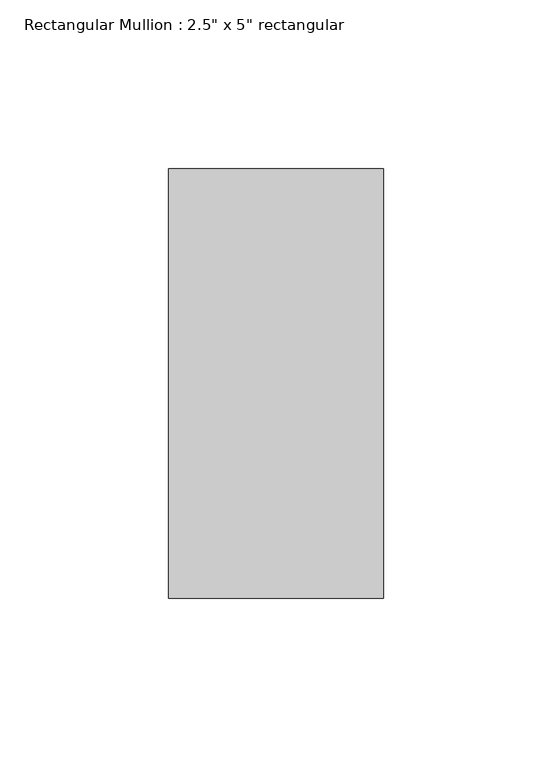
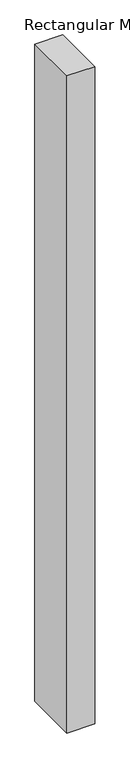
"""IFC4 building model written with IfcOpenShell, lengths in millimetres: member geometry."""

from ifc_helpers import new_model, si_unit, frame, origin, place, context, project, spatial, polyline, outline, extrude, source, transform, mapped, element, save


def member_46fa6ebc(model_context):
    return source(origin(), model_context, "Body", "SweptSolid", [
        extrude(outline(polyline([(31.75, 63.5), (31.75, -63.5), (-31.75, -63.5), (-31.75, 63.5), (31.75, 63.5)])), frame((0.0, 0.0, -1588.1134655), z_axis=(0.0, 0.0, 1.0), x_axis=(1.0, 0.0, 0.0)), (0.0, 0.0, 1.0), 1588.1134655),
    ])


if __name__ == "__main__":
    model = new_model("IFC4")
    model_context = context("Model", 3, world=origin())
    ifc_project = project(units=[si_unit("LENGTHUNIT", "METRE", prefix="MILLI")], contexts=[model_context])
    site = spatial("IfcSite", under=ifc_project)
    building = spatial("IfcBuilding", under=site)
    placement = place(None, origin())
    member_shape = member_46fa6ebc(model_context)
    element("IfcMember", 1, ObjectType="Rectangular Mullion : 2.5\" x 5\" rectangular", at=placement, inside=building, context=model_context, shape_type="MappedRepresentation", body=[
        mapped(member_shape, transform((0.0, 0.0, 0.0), x_axis=(1.0, 0.0, 0.0), y_axis=(0.0, 1.0, 0.0), z_axis=(0.0, 0.0, 1.0))),
    ])
    save(model, "model.ifc")

# Revit data of these elements
# Type "Rectangular Mullion : 2.5\" x 5\" rectangular"
#   built-in parameter 1007304 = 0.416667 (stored number, unit not read)
#   built-in parameter 1007301 = 0.104167 (stored number, unit not read)
#   built-in parameter 1007300 = 0.104167 (stored number, unit not read)
# Element 1 (IfcMember, "Rectangular Mullion : 2.5\" x 5\" rectangular")
#   Materials on its faces: "Aluminum"
# Materials
#   "Aluminum": class "Metal", colour RGB 247 247 247, transparency 0, Description = "Aluminum 6061", Cost = 0
